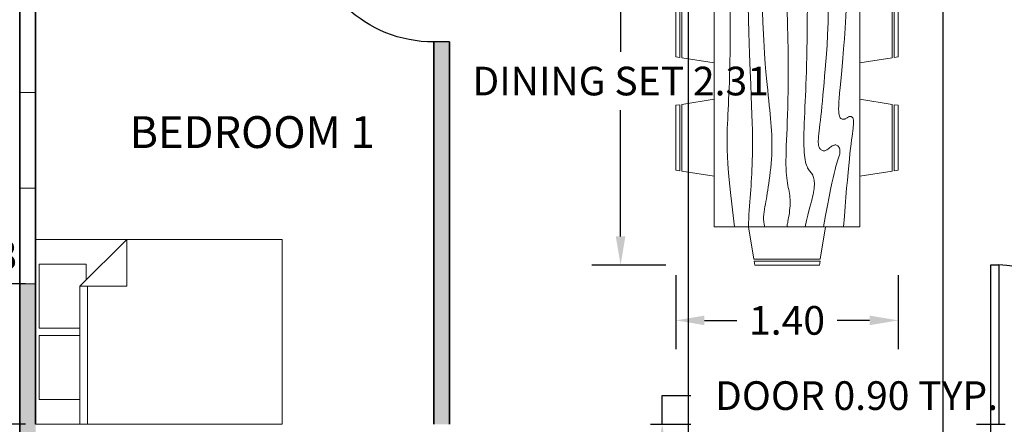
# Model space of a CAD drawing. Units: metres. Extents: x -1.9 to 13.1, y 0.9 to 14.8.
# Tile 3 of 7: x 1.2 to 7.4, y 5.9 to 8.4. Entities that reach past the tile are written whole.
import ezdxf

# ---------------------------------------------------------------- set-up
doc = ezdxf.new("R2010")
doc.units = ezdxf.units.M
doc.header["$MEASUREMENT"] = 0
for name, color, linetype, lineweight in [('A-ANNO-DIMS', 2, 'Continuous', 13), ('A-AREA-IDEN', 7, 'Continuous', 25), ('A-DOOR', 3, 'Continuous', 25), ('A-FURN', 8, 'Continuous', 18), ('A-GLAZ', 4, 'Continuous', 18), ('A-WALL', 7, 'Continuous', 35), ('A-WALL-PATT', 252, 'Continuous', 13)]:
    doc.layers.add(name, color=color, linetype=linetype, lineweight=lineweight)
doc.styles.get("Standard").update_dxf_attribs({"font": 'arial.ttf'})
doc.dimstyles.get("Standard").update_dxf_attribs({"dimtxt": 0.18, "dimasz": 0.18, "dimexe": 0.18, "dimexo": 0.0625, "dimgap": 0.09, "dimtad": 0, "dimtih": 1, "dimtoh": 1, "dimzin": 0, "dimdsep": 46, "dimlunit": 3, "dimtxsty": 'Standard', "dimcen": 0.09, "dimadec": 0, "dimazin": 0, "dimtfac": 1, "dimtofl": 0, "dimtmove": 0, "dimatfit": 3, "dimfxl": 1, "dimtolj": 1, "dimtzin": 0, "dimarcsym": 0})

# ---------------------------------------------------------------- blocks, each defined once
blk = doc.blocks.new('Dining Set - 36 x 72 in.')
for p, q in [((-22, 27.5), (-22.1562, 26.50042)), ((-22, 27.5), (-6, 27.5)), ((-5.8437, 26.49966), (-6, 27.5)), ((6, 27.5), (5.8438, 26.50042)), ((6, 27.5), (22, 27.5)), ((22.1563, 26.49966), (22, 27.5)), ((-22.2343, 26.00059), (-23.4847, 17.99762)), ((-22.2304, 26), (-5.7608, 26)), ((-5.8416, 26.5), (-22.1534, 26.5)), ((-4.5152, 17.99762), (-5.7655, 25.99926)), ((5.7657, 26.00059), (4.5153, 17.99762)), ((5.7696, 26), (22.2392, 26)), ((22.1584, 26.5), (5.8466, 26.5)), ((23.4848, 17.99762), (22.2345, 25.99926)), ((36, 18), (-36, 18)), ((-36, 18), (-36, -18)), ((36, -18), (36, 18)), ((-45.5, 8), (-44.5004, 8.15617)), ((-45.5, 8), (-45.5, -8)), ((-44.5, -8.15843), (-44.5, 8.15338)), ((-44.0006, 8.23428), (-35.9976, 9.48474)), ((-44, 8.23041), (-44, -8.23915)), ((44.0006, 8.23428), (35.9976, 9.48474)), ((44, 8.23041), (44, -8.23915)), ((44.5, -8.15843), (44.5, 8.15338)), ((45.5, 8), (44.5005, 8.15617)), ((45.5, 8), (45.5, -8)), ((-44.4997, -8.15631), (-45.5, -8)), ((-35.9976, -9.48476), (-43.9993, -8.2345)), ((35.9976, -9.48476), (43.9993, -8.2345)), ((44.4997, -8.15631), (45.5, -8)), ((-36, -18), (36, -18)), ((-22.2343, -26.0006), (-23.4847, -17.99762)), ((-4.5152, -17.99762), (-5.7655, -25.99928)), ((5.7657, -26.0006), (4.5153, -17.99762)), ((23.4848, -17.99762), (22.2345, -25.99928)), ((-22.2304, -26), (-5.7608, -26)), ((-22, -27.5), (-22.1562, -26.50044)), ((-5.8416, -26.5), (-22.1534, -26.5)), ((-5.8437, -26.49967), (-6, -27.5)), ((5.7696, -26), (22.2392, -26)), ((6, -27.5), (5.8438, -26.50044)), ((22.1584, -26.5), (5.8466, -26.5)), ((22.1563, -26.49967), (22, -27.5)), ((-22, -27.5), (-6, -27.5)), ((6, -27.5), (22, -27.5))]:
    blk.add_line(p, q)
for points in [[(-36, 15), (-31.1772, 14.97754), (-26.8079, 14.91406), (-22.8538, 14.81543), (-19.276, 14.6875), (-16.0362, 14.53613), (-13.0957, 14.36718), (-10.4159, 14.18652), (-7.9583, 14), (-5.6904, 13.81315), (-3.6035, 13.63021), (-1.6954, 13.45508), (0.0365, 13.29166), (1.5945, 13.14388), (2.9811, 13.01562), (4.1988, 12.9108), (5.25, 12.83333), (6.1393, 12.78613), (6.8802, 12.76823), (7.4883, 12.77767), (7.9792, 12.8125), (8.3685, 12.87077), (8.6719, 12.95052), (8.9049, 13.0498), (9.0833, 13.16666), (9.2205, 13.29899), (9.3216, 13.44401), (9.3895, 13.59879), (9.4271, 13.76041), (9.4373, 13.92594), (9.4232, 14.09245), (9.3875, 14.257), (9.3333, 14.41666), (9.2638, 14.56917), (9.1836, 14.71484), (9.0975, 14.85465), (9.0104, 14.98958), (8.9272, 15.1206), (8.8529, 15.2487), (8.7922, 15.37483), (8.75, 15.5), (8.7305, 15.62467), (8.7344, 15.74739), (8.7617, 15.86621), (8.8125, 15.97916), (8.8867, 16.08431), (8.9844, 16.17968), (9.1055, 16.26334), (9.25, 16.33333), (9.4189, 16.38802), (9.6172, 16.42708), (9.8506, 16.45052), (10.125, 16.45833), (10.4463, 16.45052), (10.8203, 16.42708), (11.2529, 16.38802), (11.75, 16.33333), (12.3184, 16.26318), (12.9694, 16.17838), (13.7151, 16.07991), (14.5677, 15.96875), (15.5395, 15.84586), (16.6426, 15.71224), (17.8893, 15.56884), (19.2917, 15.41666), (20.859, 15.25667), (22.5879, 15.08984), (24.4721, 14.91715), (26.5052, 14.73958), (28.6809, 14.5581), (30.9929, 14.3737), (33.4347, 14.18733), (36, 14)], [(-36, 10), (-28.9766, 10.14274), (-23.1725, 10.20442), (-18.4241, 10.19775), (-14.5677, 10.13541), (-11.4399, 10.03011), (-8.877, 9.89453), (-6.7154, 9.74137), (-4.7917, 9.58333), (-2.9698, 9.43082), (-1.2246, 9.28515), (0.4415, 9.14534), (2.026, 9.01041), (3.5266, 8.87939), (4.9408, 8.7513), (6.266, 8.62516), (7.5, 8.5), (8.6411, 8.37549), (9.6914, 8.2539), (10.6538, 8.13818), (11.5312, 8.03125), (12.3267, 7.93603), (13.043, 7.85547), (13.6831, 7.79248), (14.25, 7.75), (14.7471, 7.7303), (15.1797, 7.73307), (15.5537, 7.75732), (15.875, 7.80208), (16.1494, 7.86637), (16.3828, 7.94922), (16.5811, 8.04964), (16.75, 8.16666), (16.8944, 8.29915), (17.0143, 8.44531), (17.1089, 8.60319), (17.1771, 8.77083), (17.218, 8.94629), (17.2305, 9.1276), (17.2137, 9.31282), (17.1667, 9.5), (17.0895, 9.6875), (16.987, 9.875), (16.8649, 10.0625), (16.7292, 10.25), (16.5856, 10.4375), (16.4401, 10.625), (16.2985, 10.8125), (16.1667, 11), (16.05, 11.18733), (15.9518, 11.3737), (15.8752, 11.5581), (15.8229, 11.73958), (15.798, 11.91715), (15.8034, 12.08984), (15.842, 12.25667), (15.9167, 12.41666), (16.0295, 12.56836), (16.1784, 12.70833), (16.3605, 12.83268), (16.5729, 12.9375), (16.8127, 13.01888), (17.0768, 13.07291), (17.3625, 13.0957), (17.6667, 13.08333), (17.9894, 13.03312), (18.3418, 12.94726), (18.7382, 12.82918), (19.1927, 12.68229), (19.7195, 12.51001), (20.3327, 12.31575), (21.0465, 12.10294), (21.875, 11.875), (22.8357, 11.63354), (23.959, 11.37304), (25.2786, 11.08618), (26.8282, 10.76562), (28.6414, 10.40405), (30.752, 9.99414), (33.1936, 9.52856), (36, 9)], [(-36, 5.5), (-30.7157, 5.3348), (-26.069, 5.20963), (-21.9946, 5.11767), (-18.4271, 5.05208), (-15.3009, 5.00602), (-12.5508, 4.97265), (-10.1112, 4.94515), (-7.9167, 4.91666), (-5.909, 4.88167), (-4.0586, 4.83984), (-2.3429, 4.79215), (-0.7396, 4.73958), (0.7739, 4.6831), (2.22, 4.6237), (3.6213, 4.56233), (5, 4.5), (6.373, 4.43782), (7.7344, 4.3776), (9.0723, 4.32129), (10.375, 4.27083), (11.6309, 4.22819), (12.8281, 4.19531), (13.9551, 4.17415), (15, 4.16666), (15.954, 4.17448), (16.819, 4.19791), (17.6001, 4.23698), (18.3021, 4.29166), (18.9299, 4.36198), (19.4883, 4.44791), (19.9823, 4.54948), (20.4167, 4.66666), (20.7969, 4.79899), (21.1302, 4.94401), (21.4245, 5.09879), (21.6875, 5.26041), (21.9271, 5.42594), (22.1511, 5.59245), (22.3672, 5.757), (22.5834, 5.91666), (22.8065, 6.06868), (23.0404, 6.21093), (23.2879, 6.34147), (23.5521, 6.45833), (23.8358, 6.55957), (24.142, 6.64323), (24.4735, 6.70735), (24.8334, 6.75), (25.2235, 6.76969), (25.642, 6.76692), (26.0858, 6.74267), (26.5521, 6.69791), (27.0379, 6.63362), (27.5404, 6.55078), (28.0565, 6.45036), (28.5834, 6.33333), (29.1242, 6.19987), (29.7071, 6.04687), (30.3661, 5.87044), (31.1354, 5.66666), (32.0493, 5.43164), (33.142, 5.16146), (34.4475, 4.85221), (36, 4.5)], [(-36, -1), (-30.7915, -0.6591), (-26.0195, -0.38216), (-21.6519, -0.16284), (-17.6563, 0.00521), (-14.0005, 0.12833), (-10.6523, 0.21289), (-7.5796, 0.26522), (-4.75, 0.29166), (-2.134, 0.29793), (0.2878, 0.28711), (2.5317, 0.26163), (4.6146, 0.22396), (6.5529, 0.17651), (8.3633, 0.12174), (10.0623, 0.06209), (11.6667, 0), (13.1899, -0.06201), (14.6341, -0.1211), (15.9982, -0.17432), (17.2813, -0.21875), (18.4823, -0.25147), (19.6003, -0.26953), (20.6343, -0.27002), (21.5834, -0.25), (22.4481, -0.20768), (23.2357, -0.14584), (23.9549, -0.06836), (24.6146, 0.02083), (25.2235, 0.11784), (25.7904, 0.21875), (26.3241, 0.31966), (26.8334, 0.41666), (27.3265, 0.50618), (27.8099, 0.58593), (28.2894, 0.65397), (28.7709, 0.70833), (29.2601, 0.74707), (29.763, 0.76823), (30.2855, 0.76985), (30.8334, 0.75), (31.4088, 0.70784), (31.9994, 0.64713), (32.589, 0.57275), (33.1615, 0.48958), (33.7008, 0.4025), (34.1908, 0.3164), (34.6153, 0.23616), (34.9584, 0.16666), (35.2099, 0.11165), (35.3848, 0.07031), (35.504, 0.04069), (35.5886, 0.02083), (35.6594, 0.00879), (35.7377, 0.0026), (35.8442, 0.00032), (36, 0)], [(-36, -6.5), (-27.1843, -6.31267), (-20.084, -6.1263), (-14.469, -5.9419), (-10.1094, -5.76042), (-6.7752, -5.58285), (-4.2363, -5.41016), (-2.2629, -5.24333), (-0.625, -5.08334), (0.8708, -4.93099), (2.2715, -4.78646), (3.5872, -4.64974), (4.8281, -4.52084), (6.0046, -4.39974), (7.127, -4.28646), (8.2053, -4.18099), (9.25, -4.08334), (10.2705, -3.99382), (11.2734, -3.91407), (12.2647, -3.84603), (13.25, -3.79167), (14.2354, -3.75293), (15.2266, -3.73177), (16.2295, -3.73015), (17.25, -3.75), (18.2912, -3.79248), (19.3451, -3.85547), (20.4009, -3.93604), (21.4479, -4.03125), (22.4754, -4.13819), (23.4727, -4.25391), (24.4289, -4.37549), (25.3334, -4.5), (26.1785, -4.62492), (26.9694, -4.74935), (27.7145, -4.87281), (28.4219, -4.99479), (29.1, -5.11483), (29.7572, -5.23242), (30.4016, -5.34709), (31.0417, -5.45834), (31.6837, -5.56437), (32.3262, -5.65821), (32.9658, -5.73153), (33.599, -5.77604), (34.2224, -5.78345), (34.8327, -5.74545), (35.4264, -5.65373), (36, -5.5)], [(-36, -10), (-26.4022, -9.81299), (-18.4675, -9.62891), (-11.9839, -9.45069), (-6.7396, -9.28125), (-2.5226, -9.12354), (0.8789, -8.98047), (3.6769, -8.85498), (6.0833, -8.75), (8.2767, -8.66765), (10.3021, -8.60677), (12.1712, -8.56543), (13.8958, -8.54167), (15.4876, -8.53353), (16.9583, -8.53907), (18.3197, -8.55632), (19.5834, -8.58334), (20.7616, -8.61841), (21.8685, -8.66081), (22.9188, -8.71004), (23.9271, -8.76563), (24.9081, -8.82707), (25.8763, -8.89388), (26.8465, -8.96558), (27.8334, -9.04167), (28.8474, -9.12118), (29.8828, -9.20117), (30.93, -9.27824), (31.9792, -9.34896), (33.0205, -9.40991), (34.0443, -9.45768), (35.0407, -9.48885), (36, -9.5)], [(-36, -14.5), (-30.0881, -14.33513), (-25.0332, -14.21224), (-20.7312, -14.12647), (-17.0781, -14.07292), (-13.97, -14.04671), (-11.3027, -14.04297), (-8.9724, -14.05681), (-6.875, -14.08334), (-4.9224, -14.11833), (-3.0905, -14.16016), (-1.3709, -14.20785), (0.2448, -14.26042), (1.7647, -14.3169), (3.1973, -14.3763), (4.5507, -14.43767), (5.8333, -14.5), (7.0554, -14.5621), (8.235, -14.62175), (9.3922, -14.67652), (10.5469, -14.72396), (11.7192, -14.76164), (12.929, -14.78711), (14.1965, -14.79794), (15.5417, -14.79167), (16.9933, -14.76424), (18.6152, -14.70508), (20.4804, -14.60197), (22.6615, -14.44271), (25.2312, -14.21509), (28.2624, -13.9069), (31.8277, -13.50594), (36, -13)]]:
    blk.add_lwpolyline(points)
blk = doc.blocks.new('Bed - Queen')
for p, q in [((0, -80.00003), (0, 0)), ((0, 0), (59.99999, 0)), ((59.99999, 0), (59.99999, -80.00003)), ((7.99999, -1.2), (28.79998, -1.2)), ((7.99999, -14.4), (7.99999, -1.2)), ((28.79998, -1.2), (28.79998, -14.4)), ((31.19999, -1.2), (51.99999, -1.2)), ((31.19999, -14.4), (31.19999, -1.2)), ((51.99999, -1.2), (51.99999, -16.4)), ((0, -14.4), (44.8, -14.4)), ((59.99999, -29.6), (44.8, -14.4)), ((44.8, -14.4), (44.8, -29.6)), ((44.8, -16.8), (0, -16.8)), ((51.99999, -16.4), (46.79936, -16.4)), ((44.8, -29.6), (59.99999, -29.6)), ((59.99999, -80.00003), (0, -80.00003))]:
    blk.add_line(p, q)
blk = doc.blocks.new('*D13')
at = {"layer": 'A-ANNO-DIMS', "color": 0, "lineweight": -2, "transparency": 16777216}
for p, q in [((7.1663, 13.6964), (12.9272, 13.6964)), ((12.7472, 13.5164), (12.7472, 8.3783)), ((12.7472, 2.8764), (12.7472, 8.0145)), ((10.2663, 2.6964), (12.9272, 2.6964))]:
    blk.add_line(p, q, dxfattribs=at)
at = {"layer": 'A-ANNO-DIMS', "color": 0, "transparency": 16777216}
for points in [[(12.7172, 13.5164), (12.7772, 13.5164), (12.7472, 13.6964)], [(12.7172, 2.8764), (12.7772, 2.8764), (12.7472, 2.6964)]]:
    blk.add_solid(points, dxfattribs=at)
at = {"layer": 'Defpoints', "color": 0, "transparency": 16777216}
for p in [(7.1038, 13.6964), (12.7472, 13.6964), (10.2038, 2.6964)]:
    blk.add_point(p, dxfattribs=at)
at = {"layer": 'A-ANNO-DIMS', "color": 0, "transparency": 16777216, "insert": (12.7472, 8.1964), "char_height": 0.18, "attachment_point": 5}
blk.add_mtext('\\A1;11.00"', dxfattribs=at)
blk = doc.blocks.new('*D20')
at = {"layer": 'A-ANNO-DIMS', "color": 0, "lineweight": -2, "transparency": 16777216}
for p, q in [((1.1413, 10.5964), (-1.7723, 10.5964)), ((-1.5923, 10.4164), (-1.5923, 6.8283)), ((-1.5923, 2.8764), (-1.5923, 6.4645)), ((1.1413, 2.6964), (-1.7723, 2.6964))]:
    blk.add_line(p, q, dxfattribs=at)
at = {"layer": 'A-ANNO-DIMS', "color": 0, "transparency": 16777216}
for points in [[(-1.6223, 10.4164), (-1.5623, 10.4164), (-1.5923, 10.5964)], [(-1.6223, 2.8764), (-1.5623, 2.8764), (-1.5923, 2.6964)]]:
    blk.add_solid(points, dxfattribs=at)
at = {"layer": 'Defpoints', "color": 0, "transparency": 16777216}
for p in [(1.2038, 10.5964), (-1.5923, 2.6964), (1.2038, 2.6964)]:
    blk.add_point(p, dxfattribs=at)
at = {"layer": 'A-ANNO-DIMS', "color": 0, "transparency": 16777216, "insert": (-1.5923, 6.6464), "char_height": 0.18, "attachment_point": 5}
blk.add_mtext('\\A1;7.90"', dxfattribs=at)
blk = doc.blocks.new('*D22')
at = {"layer": 'A-ANNO-DIMS', "color": 0, "lineweight": -2, "transparency": 16777216}
for p, q in [((1.1413, 9.2964), (-0.3896, 9.2964)), ((-0.2096, 9.1164), (-0.2096, 7.7756)), ((-0.2096, 6.0709), (-0.2096, 7.4117)), ((1.1413, 5.8909), (-0.3896, 5.8909))]:
    blk.add_line(p, q, dxfattribs=at)
at = {"layer": 'A-ANNO-DIMS', "color": 0, "transparency": 16777216}
for points in [[(-0.2396, 9.1164), (-0.1796, 9.1164), (-0.2096, 9.2964)], [(-0.2396, 6.0709), (-0.1796, 6.0709), (-0.2096, 5.8909)]]:
    blk.add_solid(points, dxfattribs=at)
at = {"layer": 'Defpoints', "color": 0, "transparency": 16777216}
for p in [(1.2038, 9.2964), (-0.2096, 5.8909), (1.2038, 5.8909)]:
    blk.add_point(p, dxfattribs=at)
at = {"layer": 'A-ANNO-DIMS', "color": 0, "transparency": 16777216, "insert": (-0.2096, 7.5936), "char_height": 0.18, "attachment_point": 5}
blk.add_mtext('\\A1;3.41"', dxfattribs=at)
blk = doc.blocks.new('DOOR-800')
for p, q in [((0, 0.9), (0, 0.8)), ((0.8, 0.9), (0.8, 0.8)), ((0.75, 0), (0.75, 0.8)), ((0.75, 0.8), (0.8, 0.8)), ((0.8, 0.8), (0.8, 0)), ((0.8, 0), (0.75, 0))]:
    blk.add_line(p, q)
blk.add_arc((0.8017, 0.8), 0.8017, 180, 266.30478)
blk = doc.blocks.new('WIN-1800')
for p, q in [((0, 0.1), (0, 0)), ((0.6, 0.1), (0.6, 0)), ((1.2, 0.1), (1.2, 0)), ((1.8, 0.1), (1.8, 0))]:
    blk.add_line(p, q)
blk = doc.blocks.new('*D34')
at = {"layer": 'A-ANNO-DIMS', "color": 0, "lineweight": -2, "transparency": 16777216}
for p, q in [((5.2388, 5.8964), (5.2388, 6.0764)), ((5.2388, 6.0764), (5.4188, 6.0764)), ((5.1663, 5.8964), (5.4188, 5.8964)), ((5.2388, 5.1764), (5.2388, 5.7164)), ((5.1663, 4.9964), (5.4188, 4.9964))]:
    blk.add_line(p, q, dxfattribs=at)
at = {"layer": 'A-ANNO-DIMS', "color": 0, "transparency": 16777216}
for points in [[(5.2088, 5.7164), (5.2688, 5.7164), (5.2388, 5.8964)], [(5.2088, 5.1764), (5.2688, 5.1764), (5.2388, 4.9964)]]:
    blk.add_solid(points, dxfattribs=at)
at = {"layer": 'Defpoints', "color": 0, "transparency": 16777216}
for p in [(5.1038, 5.8964), (5.2388, 5.8964), (5.1038, 4.9964)]:
    blk.add_point(p, dxfattribs=at)
at = {"layer": 'A-ANNO-DIMS', "color": 0, "transparency": 16777216, "insert": (6.4594, 6.0764), "char_height": 0.18, "attachment_point": 5}
blk.add_mtext('\\A1;DOOR 0.90 TYP.', dxfattribs=at)
blk = doc.blocks.new('*D44')
at = {"layer": 'A-ANNO-DIMS', "color": 0, "lineweight": -2, "transparency": 16777216}
for p, q in [((5.262, 9.2068), (4.7978, 9.2068)), ((4.9778, 9.0268), (4.9778, 8.2342)), ((4.9778, 7.0754), (4.9778, 7.8679)), ((5.262, 6.8954), (4.7978, 6.8954))]:
    blk.add_line(p, q, dxfattribs=at)
at = {"layer": 'A-ANNO-DIMS', "color": 0, "transparency": 16777216}
for points in [[(4.9478, 9.0268), (5.0078, 9.0268), (4.9778, 9.2068)], [(4.9478, 7.0754), (5.0078, 7.0754), (4.9778, 6.8954)]]:
    blk.add_solid(points, dxfattribs=at)
at = {"layer": 'Defpoints', "color": 0, "transparency": 16777216}
for p in [(5.3245, 9.2068), (4.9778, 6.8954), (5.3245, 6.8954)]:
    blk.add_point(p, dxfattribs=at)
at = {"layer": 'A-ANNO-DIMS', "color": 0, "transparency": 16777216, "insert": (4.9778, 8.0511), "char_height": 0.18, "attachment_point": 5}
blk.add_mtext('\\A1;DINING SET 2.31', dxfattribs=at)
blk = doc.blocks.new('*D45')
at = {"layer": 'A-ANNO-DIMS', "color": 0, "lineweight": -2, "transparency": 16777216}
for p, q in [((5.3245, 6.8329), (5.3245, 6.3687)), ((6.7215, 6.8329), (6.7215, 6.3687)), ((5.5045, 6.5487), (5.708, 6.5487)), ((6.5415, 6.5487), (6.338, 6.5487))]:
    blk.add_line(p, q, dxfattribs=at)
at = {"layer": 'A-ANNO-DIMS', "color": 0, "transparency": 16777216}
for points in [[(5.5045, 6.5787), (5.5045, 6.5187), (5.3245, 6.5487)], [(6.5415, 6.5787), (6.5415, 6.5187), (6.7215, 6.5487)]]:
    blk.add_solid(points, dxfattribs=at)
at = {"layer": 'Defpoints', "color": 0, "transparency": 16777216}
for p in [(5.3245, 6.8954), (6.7215, 6.8954), (6.7215, 6.5487)]:
    blk.add_point(p, dxfattribs=at)
at = {"layer": 'A-ANNO-DIMS', "color": 0, "transparency": 16777216, "insert": (6.023, 6.5487), "char_height": 0.18, "attachment_point": 5}
blk.add_mtext('\\A1;1.40', dxfattribs=at)
blk = doc.blocks.new('*D52')
at = {"layer": 'A-ANNO-DIMS', "color": 0, "lineweight": -2, "transparency": 16777216}
for p, q in [((0.4443, 6.7785), (0.4443, 6.9585)), ((0.4443, 6.9585), (0.6243, 6.9585)), ((1.2413, 6.7785), (0.2643, 6.7785)), ((0.4443, 6.0764), (0.4443, 6.5985)), ((1.2413, 5.8964), (0.2643, 5.8964))]:
    blk.add_line(p, q, dxfattribs=at)
at = {"layer": 'A-ANNO-DIMS', "color": 0, "transparency": 16777216}
for points in [[(0.4143, 6.5985), (0.4743, 6.5985), (0.4443, 6.7785)], [(0.4143, 6.0764), (0.4743, 6.0764), (0.4443, 5.8964)]]:
    blk.add_solid(points, dxfattribs=at)
at = {"layer": 'Defpoints', "color": 0, "transparency": 16777216}
for p in [(0.4443, 6.7785), (1.3038, 6.7785), (1.3038, 5.8964)]:
    blk.add_point(p, dxfattribs=at)
at = {"layer": 'A-ANNO-DIMS', "color": 0, "transparency": 16777216, "insert": (0.9483, 6.9585), "char_height": 0.18, "attachment_point": 5}
blk.add_mtext('\\A1;0.88', dxfattribs=at)
blk = doc.blocks.new('*D66')
at = {"layer": 'A-ANNO-DIMS', "color": 0, "lineweight": -2, "transparency": 16777216}
for p, q in [((5.403847, 4.558878), (5.403847, 14.635878)), ((7.003847, 4.558878), (7.003847, 14.635878)), ((5.583847, 14.455878), (5.888847, 14.455878)), ((6.823847, 14.455878), (6.518847, 14.455878))]:
    blk.add_line(p, q, dxfattribs=at)
at = {"layer": 'A-ANNO-DIMS', "color": 0, "transparency": 16777216}
for points in [[(5.583847, 14.485878), (5.583847, 14.425878), (5.403847, 14.455878)], [(6.823847, 14.485878), (6.823847, 14.425878), (7.003847, 14.455878)]]:
    blk.add_solid(points, dxfattribs=at)
at = {"layer": 'Defpoints', "color": 0, "transparency": 16777216}
for p in [(7.003847, 14.455878), (5.403847, 4.496378), (7.003847, 4.496378)]:
    blk.add_point(p, dxfattribs=at)
at = {"layer": 'A-ANNO-DIMS', "color": 0, "transparency": 16777216, "insert": (6.203847, 14.455878), "char_height": 0.18, "attachment_point": 5}
blk.add_mtext('\\A1;1.60', dxfattribs=at)
blk = doc.blocks.new('*D75')
at = {"layer": 'A-ANNO-DIMS', "color": 0, "lineweight": -2, "transparency": 16777216}
for p, q in [((8.4637, 7.0002), (8.1587, 6.7103)), ((8.6437, 7.0002), (8.4637, 7.0002)), ((7.3025, 5.8064), (7.3025, 5.9864)), ((7.2125, 5.8964), (7.3925, 5.8964))]:
    blk.add_line(p, q, dxfattribs=at)
at = {"layer": 'A-ANNO-DIMS', "color": 0, "transparency": 16777216}
blk.add_solid([(8.1381, 6.732), (8.1794, 6.6885), (8.0283, 6.5863)], dxfattribs=at)
at = {"layer": 'Defpoints', "color": 0, "transparency": 16777216}
for p in [(8.0283, 6.5863), (7.3025, 5.8964)]:
    blk.add_point(p, dxfattribs=at)
at = {"layer": 'A-ANNO-DIMS', "color": 0, "transparency": 16777216, "insert": (9.0533, 7.0002), "char_height": 0.18, "attachment_point": 5}
blk.add_mtext('\\A1;R1.00', dxfattribs=at)

msp = doc.modelspace()

# ---------------------------------------------------------------- linework, layer by layer
at = {"layer": 'A-DOOR'}
for p, q in [((7.3038, 5.8964), (7.3038, 6.8964)), ((7.3038, 6.8964), (7.3538, 6.8964)), ((7.3538, 6.8964), (7.3538, 5.8964))]:
    msp.add_line(p, q, dxfattribs=at)
msp.add_arc((7.3025, 5.8964), 1.0013, 0, 87.0624, dxfattribs=at)
at = {"layer": 'A-WALL'}
for p, q in [((1.3038, 9.2964), (1.3038, 5.8964)), ((3.8038, 8.2964), (3.8038, 5.8964)), ((3.9038, 8.2964), (3.9038, 5.8964))]:
    msp.add_line(p, q, dxfattribs=at)
msp.add_lwpolyline([(1.2038, 10.5964), (1.2038, 2.6964), (10.2038, 2.6964), (10.2038, 10.5964)], dxfattribs=at)
at = {"layer": 'A-WALL-PATT'}
for points in [[(3.8038, 5.8964), (3.9038, 5.8964), (3.8038, 8.2964), (3.9038, 8.2964)], [(1.2038, 4.7964), (1.3038, 4.7964), (1.2038, 6.7785), (1.3038, 6.7785)]]:
    msp.add_solid(points, dxfattribs=at)

# ---------------------------------------------------------------- block references
at = {"layer": 'A-DOOR', "extrusion": (0, 0, -1), "zscale": -1, "rotation": 89.99999999999893}
msp.add_blockref('DOOR-800', (-3.0038, 8.2964), dxfattribs=at)
at = {"layer": 'A-FURN'}
for name, p, xscale, yscale, zscale, rotation in [('Dining Set - 36 x 72 in.', (6.023, 8.0511), 0.0254, 0.0254, 0.0254, 270), ('Bed - Queen', (1.3038, 5.8964), 0.0193482099346659, 0.0193482099346659, 0.0193482099346659, 90)]:
    msp.add_blockref(name, p, dxfattribs=dict(at, xscale=xscale, yscale=yscale, zscale=zscale, rotation=rotation))
at = {"layer": 'A-GLAZ', "rotation": 90.00000000000006}
msp.add_blockref('WIN-1800', (1.3038, 6.7785), dxfattribs=at)

# ---------------------------------------------------------------- texts
at = {"layer": 'A-AREA-IDEN', "insert": (1.8536, 7.8306), "char_height": 0.2, "attachment_point": 1}
msp.add_mtext_dynamic_manual_height_columns('\\pxqc;BEDROOM 1', width=1.619642, gutter_width=1, heights=[0], dxfattribs=at)

# ---------------------------------------------------------------- dimensions: what is measured, and where the dimension line sits
at = {"layer": 'A-ANNO-DIMS'}
for base, p1, p2, picture, middle in [((7.0038, 14.4559), (5.4038, 4.4964), (7.0038, 4.4964), '*D66', (6.2038, 14.4559)), ((6.7215, 6.5487), (5.3245, 6.8954), (6.7215, 6.8954), '*D45', (6.023, 6.5487))]:
    dim = msp.add_linear_dim(base=base, p1=p1, p2=p2, dimstyle='Standard', override={"dimdec": 2, "dimlfac": 1, "dimrnd": 0, "dimzin": 0, "dimdsep": 46, "dimlunit": 2}, dxfattribs=at)
    dim.commit()
    dim.dimension.update_dxf_attribs({"geometry": picture, "text_midpoint": middle})
for base, p1, p2, override, picture, middle in [((12.7472, 13.6964), (10.2038, 2.6964), (7.1038, 13.6964), {"dimclrd": 0, "dimclre": 0, "dimclrt": 0}, '*D13', (12.7472, 8.1964)), ((-1.5923, 2.6964), (1.2038, 10.5964), (1.2038, 2.6964), {"dimclrd": 0, "dimclre": 0, "dimclrt": 0}, '*D20', (-1.5923, 6.6464)), ((-0.2096, 5.8909), (1.2038, 9.2964), (1.2038, 5.8909), {"dimclrd": 0, "dimclre": 0, "dimclrt": 0}, '*D22', (-0.2096, 7.5936)), ((0.4443, 6.7785), (1.3038, 5.8964), (1.3038, 6.7785), {"dimdec": 2, "dimlfac": 1, "dimrnd": 0, "dimzin": 0, "dimdsep": 46, "dimlunit": 2}, '*D52', (0.9483, 6.9585))]:
    dim = msp.add_linear_dim(base=base, p1=p1, p2=p2, angle=90, dimstyle='Standard', override=override, dxfattribs=at)
    dim.commit()
    dim.dimension.update_dxf_attribs({"geometry": picture, "text_midpoint": middle})
for base, p1, p2, angle, text, picture, middle in [((4.9778, 6.8954), (5.3245, 9.2068), (5.3245, 6.8954), 270, 'DINING SET <>', '*D44', (4.9778, 8.0511)), ((5.2388, 5.8964), (5.1038, 4.9964), (5.1038, 5.8964), 90, 'DOOR <> TYP.', '*D34', (6.4594, 6.0764))]:
    dim = msp.add_linear_dim(base=base, p1=p1, p2=p2, angle=angle, text=text, dimstyle='Standard', override={"dimdec": 2, "dimlfac": 1, "dimrnd": 0, "dimzin": 0, "dimdsep": 46, "dimlunit": 2}, dxfattribs=at)
    dim.commit()
    dim.dimension.update_dxf_attribs({"geometry": picture, "text_midpoint": middle})
dim = msp.add_radius_dim(center=(7.3025, 5.8964), mpoint=(8.0283, 6.5863), dimstyle='Standard', override={"dimdec": 2, "dimlfac": 1, "dimrnd": 0, "dimzin": 0, "dimdsep": 46, "dimlunit": 2}, dxfattribs=at)
dim.commit()
dim.dimension.update_dxf_attribs({"geometry": '*D75', "text_midpoint": (9.0533, 7.0002), "dimtype": 164})

doc.saveas('drawing.dxf')
